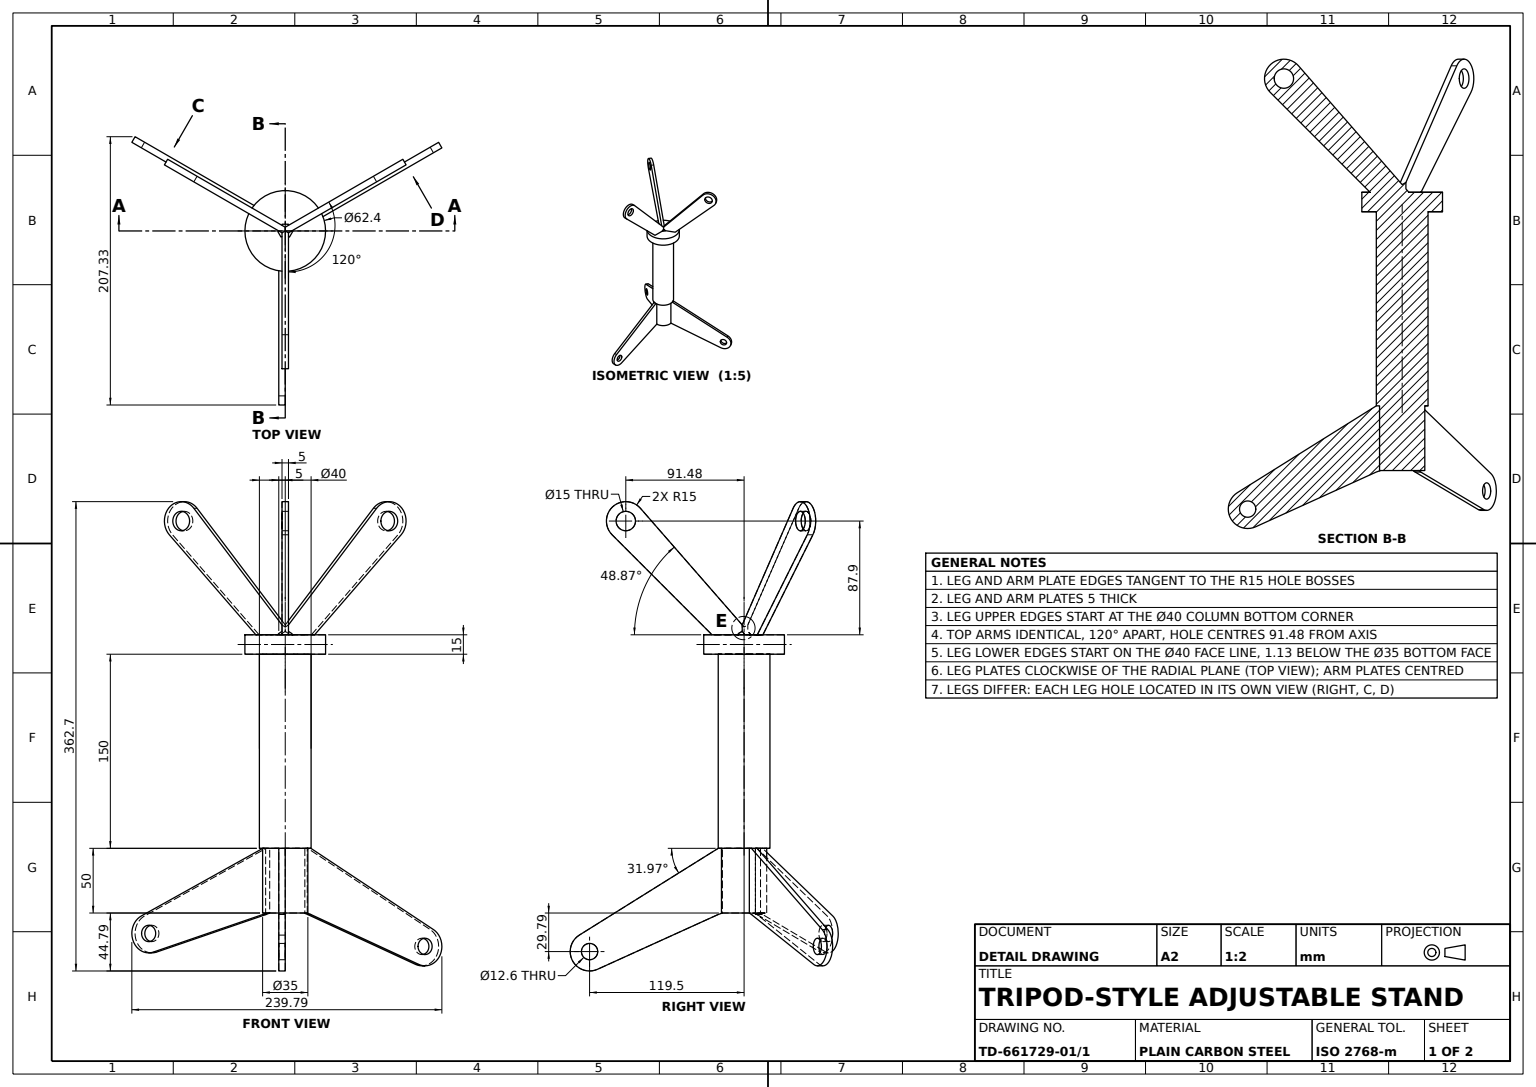
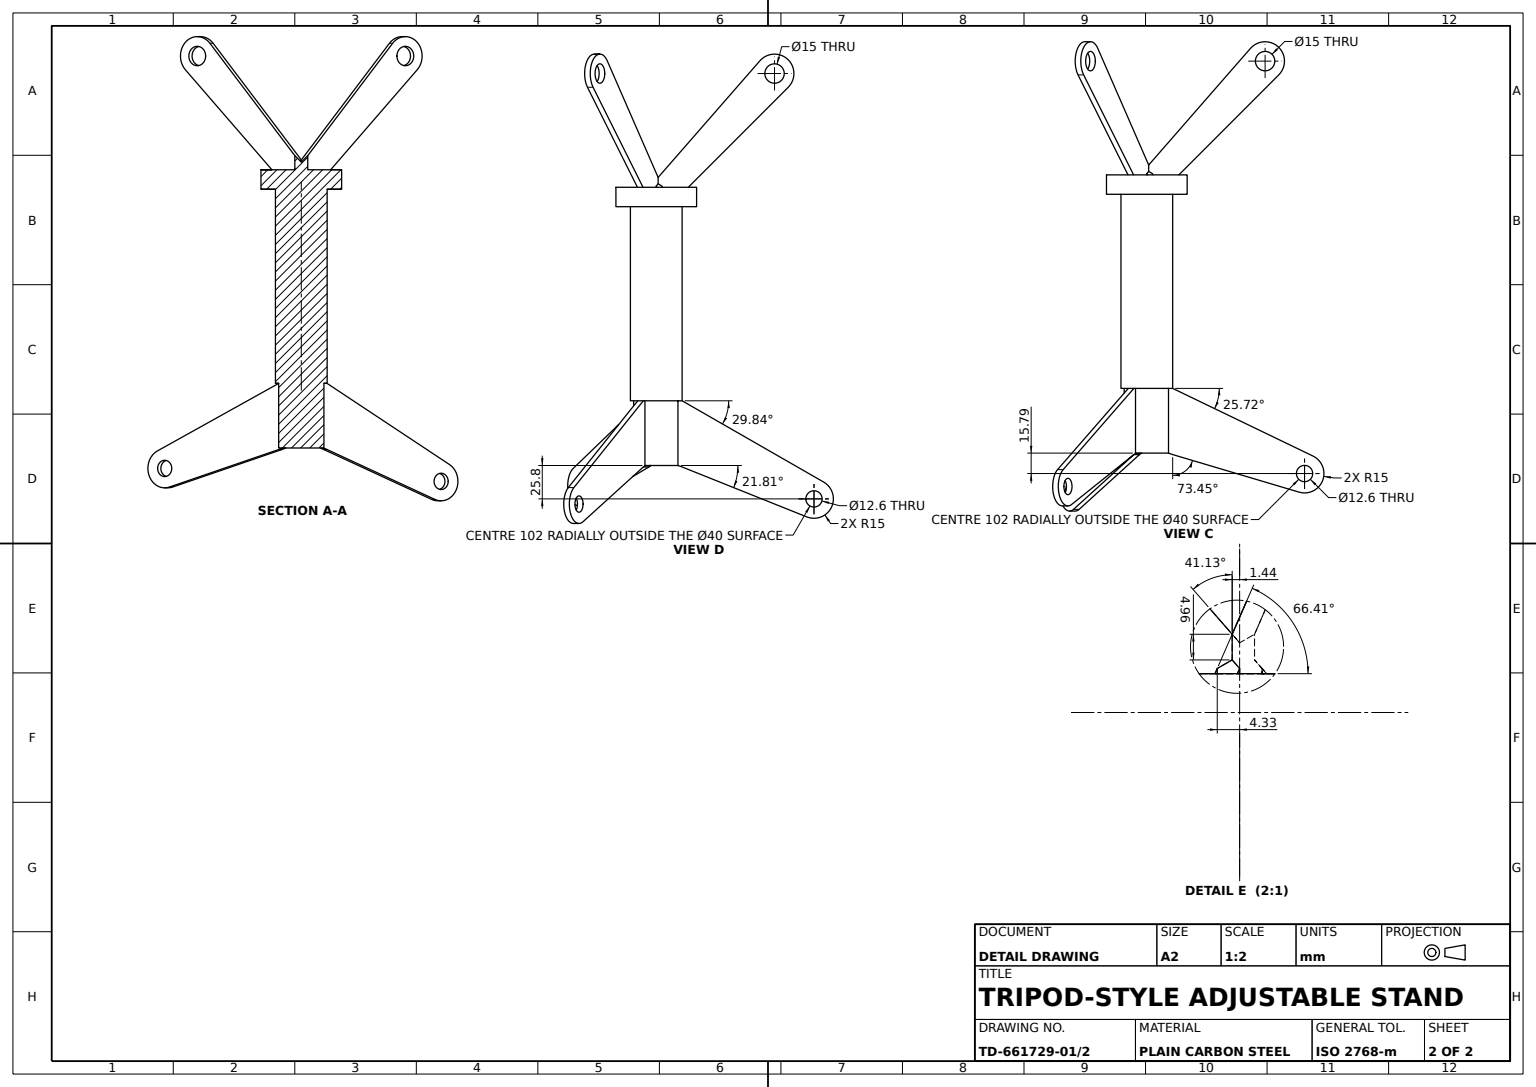
from build123d import *

# Parameters (mm, degrees)
COLUMN_SKETCH_R           = 20
COLUMN_40_DEPTH           = 150
COLUMN_EXTENSION_SKETCH_R = 17.5
COLUMN_EXTENSION_35_DEPTH = 50
LEG_PLATE_SKETCH_R        = 6.3
LEG_PLATE_DEPTH           = 5
LEG_WEB_REACH             = 191.764
LEG_WEB_END_RADIUS        = 17.5
LEG_WEB_SKETCH_W          = 5
LEG_WEB_SKETCH_H          = 51.133954969
LEG_CUT_DEPTH             = 22
LEG_WEB_PATTERN_3X_COUNT  = 3
LEG_CUT_PATTERN_3X_COUNT  = 3
LEG_BOSS_A_SKETCH_R       = 6.3
LEG_BOSS_A_DEPTH          = 5
LEG_BOSS_B_SKETCH_R       = 6.3
LEG_BOSS_B_DEPTH          = 5
COLLAR_SKETCH_R           = 31.2
COLLAR_62_4_DEPTH         = 15
TOP_ARM_SKETCH_R          = 7.5
TOP_ARM_DEPTH             = 2.5
TOP_ARM_PATTERN_3X_COUNT  = 3


with BuildPart() as part:
    # Column Sketch → Column Ø40 (new body)
    with BuildSketch(Plane(origin=(0, 0, 0), x_dir=(1, 0, 0), z_dir=(0, 1, 0))):
        with Locations(Location((0, 0, 0), (0, 0, 270))):
            Circle(COLUMN_SKETCH_R)
    extrude(amount=COLUMN_40_DEPTH)

    # Column Extension Sketch → Column Extension Ø35 (add)
    with BuildSketch(Plane.XZ):
        with Locations(Location((0, 0, 0), (0, 0, 270))):
            Circle(COLUMN_EXTENSION_SKETCH_R)
    extrude(amount=COLUMN_EXTENSION_35_DEPTH)



with BuildPart() as body_2:
    # Leg Plate Sketch → Leg Plate (new body)
    with BuildSketch(Plane.XY):
        with BuildLine():
            Line((20, 0), (127.443020473, -67.070132718))
            ThreePointArc((127.443020473, -67.070132718), (132.721270407, -86.87951221), (113.303865545, -93.454907759))
            Line((113.303865545, -93.454907759), (20, -51.133954969))
            Line((20, -51.133954969), (20, 0))
        make_face()
        with Locations((119.5, -79.794456895)):
            Circle(LEG_PLATE_SKETCH_R, mode=Mode.SUBTRACT)
    extrude(amount=LEG_PLATE_DEPTH)


with BuildPart() as part_1:
    add(part.part)

    add(body_2.part)  # Leg Web merges body 2
    # Leg Web: up to this cylinder (the profile starts outside it)
    leg_web_end = Plane(origin=(0, -25.566977, 0), z_dir=(0, 1, 0)) * Cylinder(LEG_WEB_END_RADIUS, 419.528, mode=Mode.PRIVATE)
    # Leg Web Sketch → Leg Web (add, up to the surface)
    with BuildSketch(Plane.ZY.offset(-20), mode=Mode.PRIVATE) as leg_web_sk1:
        with Locations((2.5, -25.566977485)):
            Rectangle(LEG_WEB_SKETCH_W, LEG_WEB_SKETCH_H)
    leg_web_tool1 = extrude(leg_web_sk1.sketch, amount=LEG_WEB_REACH, mode=Mode.PRIVATE) - leg_web_end
    leg_web = leg_web_tool1.solids().sort_by_distance((20, -25.566977, 2.5))[0]
    add(leg_web)

    # Leg Cut Sketch → Leg Cut (cut)
    with BuildSketch(Plane.XY.offset(5)):
        Polygon((20, -51.133954969), (16.770509831, -50), (16.770509831, -51.133954969), align=None)
    leg_cut = extrude(amount=-LEG_CUT_DEPTH, mode=Mode.SUBTRACT)

    # Leg Web Pattern 3x: Leg Web ×3 about axis
    leg_web_pattern_3x_axis = Axis((0, 0, 0), (0, 1, 0))
    for i in range(1, LEG_WEB_PATTERN_3X_COUNT):
        add(leg_web.rotate(leg_web_pattern_3x_axis, i * 360 / LEG_WEB_PATTERN_3X_COUNT))

    # Leg Cut Pattern 3x: Leg Cut ×3 about axis
    leg_cut_pattern_3x_axis = Axis((0, 0, 0), (0, 1, 0))
    for i in range(1, LEG_CUT_PATTERN_3X_COUNT):
        add(leg_cut.rotate(leg_cut_pattern_3x_axis, i * 360 / LEG_CUT_PATTERN_3X_COUNT), mode=Mode.SUBTRACT)

    # Leg Boss A Sketch → Leg Boss A (add)
    with BuildSketch(Plane(origin=(4.330127019, 0, -2.5), x_dir=(-0.49999999999999195, 0, -0.8660254037844434), z_dir=(0.8660254037844434, 0, -0.49999999999999195))):
        with BuildLine():
            Line((20, -51.133954969), (116.426306648, -89.727235024))
            ThreePointArc((116.426306648, -89.727235024), (135.501802499, -82.335843689), (129.463513173, -62.789839753))
            Line((129.463513173, -62.789839753), (20, 0))
            Line((20, 0), (20, -51.133954969))
        make_face()
        with Locations((122, -75.801218278)):
            Circle(LEG_BOSS_A_SKETCH_R, mode=Mode.SUBTRACT)
    extrude(amount=-LEG_BOSS_A_DEPTH)

    # Leg Boss B Sketch → Leg Boss B (add)
    with BuildSketch(Plane(origin=(-4.330127019, 0, -2.5), x_dir=(-0.5000000000000041, 0, 0.8660254037844364), z_dir=(-0.8660254037844363, 0, -0.500000000000004))):
        with BuildLine():
            Line((20, -51.133954969), (117.728382424, -80.166617623))
            ThreePointArc((117.728382424, -80.166617623), (135.9911189, -71.195896344), (128.510110547, -52.274059807))
            Line((128.510110547, -52.274059807), (20, 0))
            Line((20, 0), (20, -51.133954969))
        make_face()
        with Locations((122, -65.787699608)):
            Circle(LEG_BOSS_B_SKETCH_R, mode=Mode.SUBTRACT)
    extrude(amount=-LEG_BOSS_B_DEPTH)

    # Collar Sketch → Collar Ø62.4 (add)
    with BuildSketch(Plane(origin=(0, 150, 0), x_dir=(1, 0, 0), z_dir=(0, 1, 0))):
        with Locations(Location((0, 0, 0), (0, 0, 270))):
            Circle(COLLAR_SKETCH_R)
    extrude(amount=COLLAR_62_4_DEPTH)

    # Top Arm Sketch → Top Arm (add, symmetric)
    with BuildSketch(Plane.XY):
        with BuildLine():
            Line((-5.207772038, 165), (80.183921166, 262.769823837))
            ThreePointArc((80.183921166, 262.769823837), (101.724330238, 263.860880188), (102.088153724, 242.295925762))
            Line((102.088153724, 242.295925762), (24.792227962, 165))
            Line((24.792227962, 165), (-5.207772038, 165))
        make_face()
        with Locations((91.481552006, 252.902527479)):
            Circle(TOP_ARM_SKETCH_R, mode=Mode.SUBTRACT)
    top_arm = extrude(amount=TOP_ARM_DEPTH, both=True)

    # Top Arm Pattern 3x: Top Arm ×3 about axis
    top_arm_pattern_3x_axis = Axis((0, 0, 0), (0, 1, 0))
    for i in range(1, TOP_ARM_PATTERN_3X_COUNT):
        add(top_arm.rotate(top_arm_pattern_3x_axis, i * 360 / TOP_ARM_PATTERN_3X_COUNT))


solid = part_1.part
